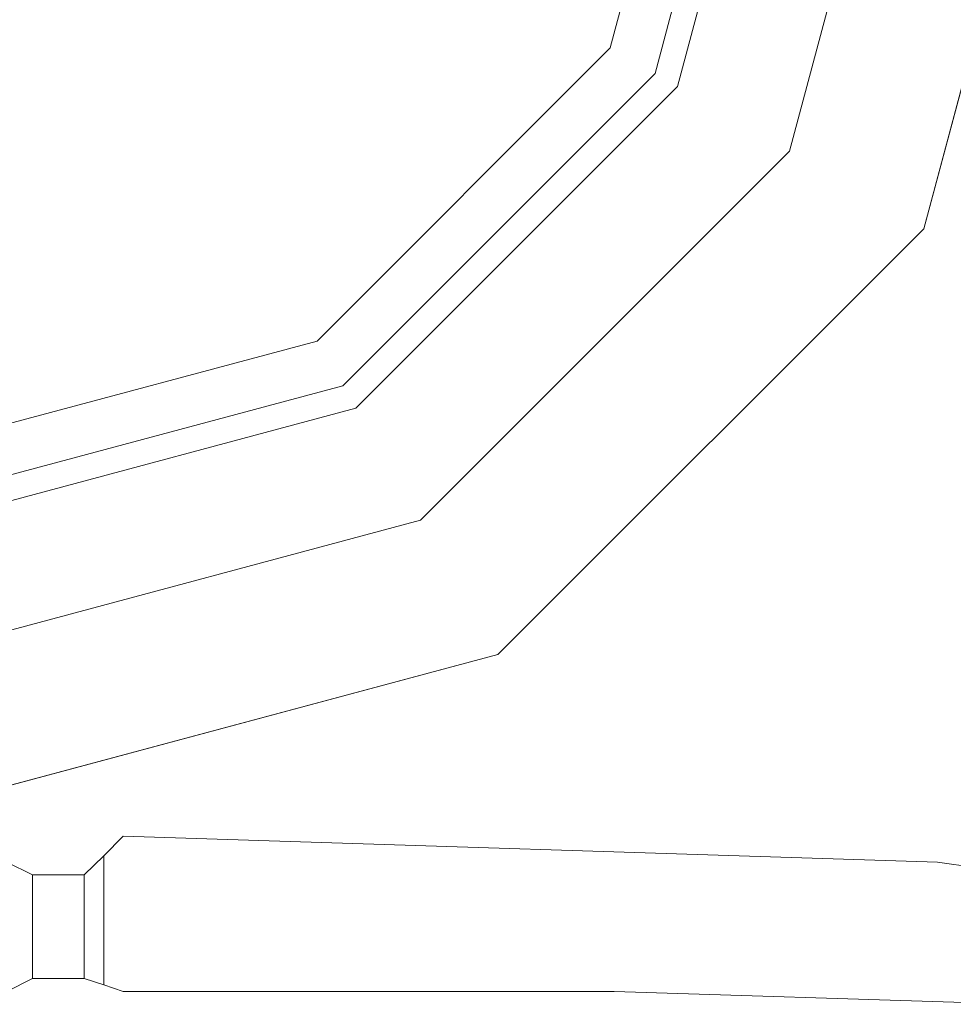
# Model space of a CAD drawing. Units: inches. Extents: x 375 to 1122, y 27 to 1069.
# Tile 19 of 155: x 713.046 to 717.492, y 270.778 to 275.466. Entities that reach past the tile are written whole.
import ezdxf

# ---------------------------------------------------------------- set-up
doc = ezdxf.new("R2010")
doc.units = ezdxf.units.IN
doc.layers.add('Furniture', color=30, linetype='Continuous', lineweight=18)

# ---------------------------------------------------------------- blocks, each defined once
blk = doc.blocks.new('A$C403C54AD')
at = {"linetype": 'ByBlock', "invisible_edges": 5}
for points in [[(1.79578, 0.81008, -0.00874), (1.78654, 0.79408, -0.00874), (1.72651, 0.81017, -0.00874), (1.72651, 0.82864, -0.00874)], [(1.77884, 0.78075, -0.02259), (1.79578, 0.81008, -0.01335), (1.72651, 0.82864, -0.01335), (1.72651, 0.79478, -0.02259)], [(1.78654, 0.79408, -0.00874), (1.7773, 0.77809, -0.01489), (1.72651, 0.7917, -0.01489), (1.72651, 0.81017, -0.00874)], [(1.81715, 0.74244, -0.02259), (1.84648, 0.75938, -0.01335), (1.79578, 0.81008, -0.01335), (1.77884, 0.78075, -0.02259)], [(1.84648, 0.75938, -0.00874), (1.83048, 0.75014, -0.00874), (1.78654, 0.79408, -0.00874), (1.79578, 0.81008, -0.00874)], [(1.77423, 0.77276, -0.03183), (1.77884, 0.78075, -0.02259), (1.72651, 0.79478, -0.02259), (1.72651, 0.78554, -0.03183)], [(1.83048, 0.75014, -0.00874), (1.81449, 0.74091, -0.01489), (1.7773, 0.77809, -0.01489), (1.78654, 0.79408, -0.00874)], [(1.7773, 0.77809, -0.01489), (1.72651, 0.69011, -0.01489), (1.72651, 0.69011, -0.01489), (1.72651, 0.7917, -0.01489)], [(1.80916, 0.73783, -0.03183), (1.81715, 0.74244, -0.02259), (1.77884, 0.78075, -0.02259), (1.77423, 0.77276, -0.03183)], [(1.81449, 0.74091, -0.01489), (1.72651, 0.69011, -0.01489), (1.72651, 0.69011, -0.01489), (1.7773, 0.77809, -0.01489)], [(1.83118, 0.69011, -0.02259), (1.86504, 0.69011, -0.01335), (1.84648, 0.75938, -0.01335), (1.81715, 0.74244, -0.02259)], [(1.86504, 0.69011, -0.00874), (1.84657, 0.69011, -0.00874), (1.83048, 0.75014, -0.00874), (1.84648, 0.75938, -0.00874)], [(1.84657, 0.69011, -0.00874), (1.8281, 0.69011, -0.01489), (1.81449, 0.74091, -0.01489), (1.83048, 0.75014, -0.00874)], [(1.82194, 0.69011, -0.03183), (1.83118, 0.69011, -0.02259), (1.81715, 0.74244, -0.02259), (1.80916, 0.73783, -0.03183)], [(1.8281, 0.69011, -0.01489), (1.72651, 0.69011, -0.01489), (1.72651, 0.69011, -0.01489), (1.81449, 0.74091, -0.01489)]]:
    blk.add_3dface(points, dxfattribs=at)
at = {"linetype": 'ByBlock'}
for points in [[(1.79578, 0.81008, -0.01335), (1.79578, 0.81008, -0.00874), (1.72651, 0.82864, -0.00874), (1.72651, 0.82864, -0.01335)], [(1.84648, 0.75938, -0.01335), (1.84648, 0.75938, -0.00874), (1.79578, 0.81008, -0.00874), (1.79578, 0.81008, -0.01335)], [(1.86504, 0.69011, -0.01335), (1.86504, 0.69011, -0.00874), (1.84648, 0.75938, -0.00874), (1.84648, 0.75938, -0.01335)]]:
    blk.add_3dface(points, dxfattribs=at)
for points, invisible_edges in [([(1.87273, 0.82248, -0.0249), (1.88813, 0.82248, -0.0249), (1.88659, 0.77323, -0.0249), (1.8712, 0.81171, -0.0249)], 5), ([(1.87273, 0.82248, -0.02644), (1.88813, 0.82248, -0.02644), (1.88659, 0.77323, -0.02644), (1.8712, 0.81171, -0.02644)], 5), ([(1.87273, 0.82248, -0.0249), (1.87273, 0.82248, -0.02644), (1.8712, 0.81171, -0.02644), (1.8712, 0.81171, -0.0249)], 5), ([(1.88659, 0.77323, -0.02644), (1.88659, 0.77323, -0.0249), (1.88813, 0.82248, -0.0249), (1.88813, 0.82248, -0.02644)], 5), ([(1.88659, 0.77323, -0.0249), (1.8712, 0.81171, -0.0249), (1.86812, 0.71474, -0.0249), (1.88659, 0.71474, -0.0249)], 5), ([(1.88659, 0.77323, -0.02644), (1.8712, 0.81171, -0.02644), (1.86812, 0.71474, -0.02644), (1.88659, 0.71474, -0.02644)], 5), ([(1.8712, 0.81171, -0.02644), (1.8712, 0.81171, -0.0249), (1.86812, 0.71474, -0.0249), (1.86812, 0.71474, -0.02644)], 5), ([(1.88659, 0.71474, -0.0249), (1.88659, 0.71474, -0.02644), (1.88659, 0.77323, -0.02644), (1.88659, 0.77323, -0.0249)], 5), ([(1.86812, 0.71474, -0.0249), (1.88659, 0.71474, -0.0249), (1.88582, 0.71243, -0.02413), (1.87043, 0.71243, -0.02413)], 1), ([(1.86812, 0.71474, -0.02644), (1.88659, 0.71474, -0.02644), (1.88582, 0.71243, -0.02721), (1.87043, 0.71243, -0.02721)], 1), ([(1.86812, 0.71474, -0.02644), (1.86812, 0.71474, -0.0249), (1.87043, 0.71243, -0.02413), (1.87043, 0.71243, -0.02721)], 5), ([(1.88582, 0.71243, -0.02721), (1.88582, 0.71243, -0.02413), (1.88659, 0.71474, -0.0249), (1.88659, 0.71474, -0.02644)], 5), ([(1.87043, 0.71243, -0.02413), (1.87043, 0.71243, -0.02721), (1.87273, 0.71012, -0.03029), (1.87273, 0.71012, -0.02105)], 5), ([(1.88505, 0.71012, -0.02105), (1.88505, 0.71012, -0.03029), (1.88582, 0.71243, -0.02721), (1.88582, 0.71243, -0.02413)], 5), ([(1.87273, 0.71012, -0.03029), (1.87273, 0.71012, -0.02105), (1.87273, 0.70396, -0.02105), (1.87273, 0.70396, -0.03029)], 1), ([(1.88505, 0.70396, -0.03029), (1.88505, 0.70396, -0.02105), (1.88505, 0.71012, -0.02105), (1.88505, 0.71012, -0.03029)], 4)]:
    blk.add_3dface(points, dxfattribs=dict(invisible_edges=invisible_edges))
for points in [[(1.87043, 0.71243, -0.02413), (1.88582, 0.71243, -0.02413), (1.88505, 0.71012, -0.02105), (1.87273, 0.71012, -0.02105)], [(1.87043, 0.71243, -0.02721), (1.88582, 0.71243, -0.02721), (1.88505, 0.71012, -0.03029), (1.87273, 0.71012, -0.03029)], [(1.88505, 0.71012, -0.02105), (1.87273, 0.71012, -0.02105), (1.87273, 0.70396, -0.02105), (1.88505, 0.70396, -0.02105)], [(1.88505, 0.71012, -0.03029), (1.87273, 0.71012, -0.03029), (1.87273, 0.70396, -0.03029), (1.88505, 0.70396, -0.03029)], [(1.87273, 0.70396, -0.02105), (1.88505, 0.70396, -0.02105), (1.88659, 0.70089, -0.01951), (1.8712, 0.70089, -0.01951)], [(1.87273, 0.70396, -0.03029), (1.88505, 0.70396, -0.03029), (1.88659, 0.70089, -0.03183), (1.8712, 0.70089, -0.03183)], [(1.87273, 0.70396, -0.02105), (1.87273, 0.70396, -0.03029), (1.8712, 0.70089, -0.03183), (1.8712, 0.70089, -0.01951)], [(1.88659, 0.70089, -0.01951), (1.88659, 0.70089, -0.03183), (1.88505, 0.70396, -0.03029), (1.88505, 0.70396, -0.02105)]]:
    blk.add_3dface(points)

msp = doc.modelspace()

# ---------------------------------------------------------------- block references
at = {"layer": 'Furniture', "xscale": 39.9918517141215, "yscale": 39.9918517141215, "zscale": 39.9918517141215, "rotation": 270}
msp.add_blockref('A$C403C54AD', (684.9549, 346.2875, 0.024), dxfattribs=at)

doc.saveas('drawing.dxf')
